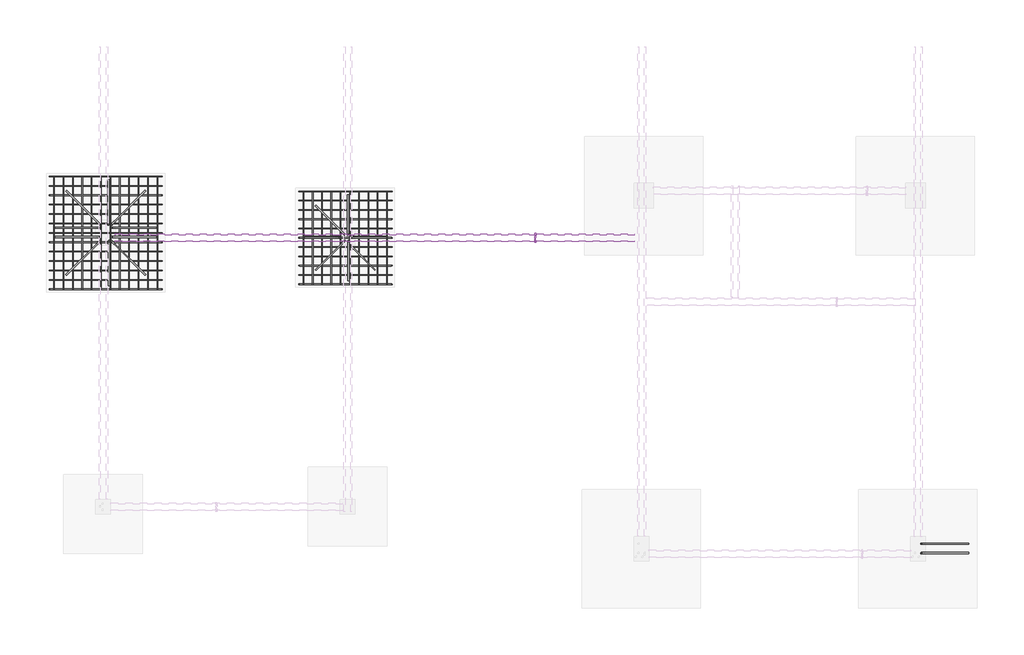
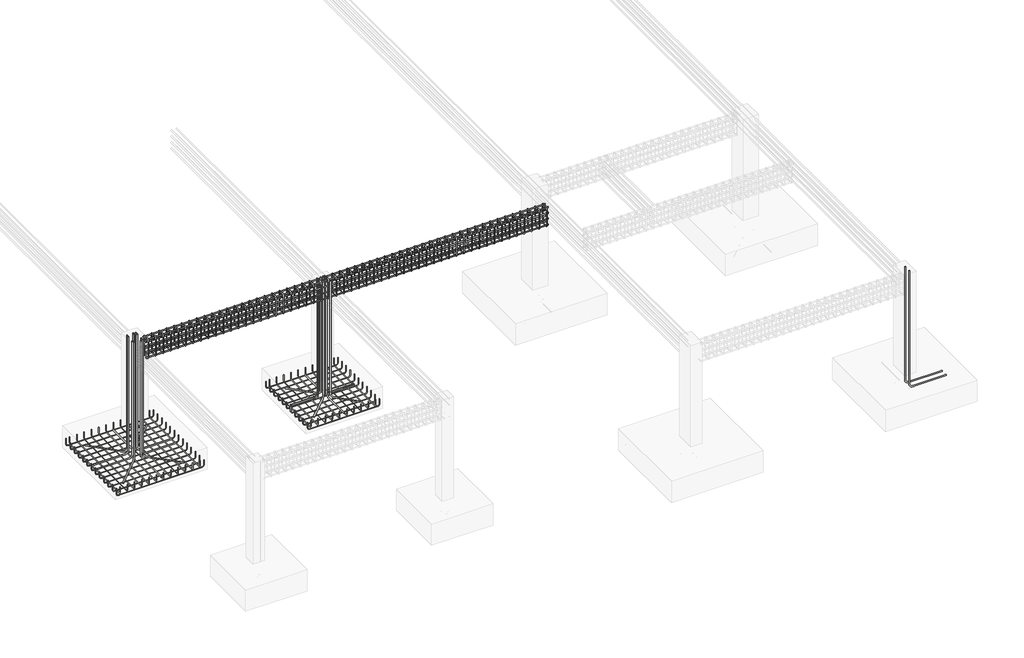
# One storey, part 4 of 10: 28 reinforcing bars.
"""IFC4 building model written with IfcOpenShell, lengths in millimetres."""

from ifc_helpers import new_model, si_unit, point, frame, origin, place, context, project, spatial, polyline, circle_curve, trimmed, segment, composite_curve, source, transform, mapped, element, save
from ifc_brep_helpers import swept_disk

model = new_model("IFC4")

# Units and contexts
model_context = context("Model", 3, world=origin())
ifc_project = project(units=[si_unit("LENGTHUNIT", "METRE", prefix="MILLI")], contexts=[model_context])

# Site, building, storey
site = spatial("IfcSite", under=ifc_project)
building = spatial("IfcBuilding", under=site)
storey = spatial("IfcBuildingStorey", under=building, Elevation=-2133.6)

# Reinforcing bars
placement = place(None, origin())
reinforcing_bar_shape = source(origin(), model_context, "Body", "SolidModel", [
    swept_disk(composite_curve([segment(polyline([(-4027.5164362, 1780.9219177, -2393.6), (-4027.5164362, 1780.9219177, -2504.1)]), True, "CONTINUOUS"), segment(trimmed(circle_curve(frame((-4062.2664362, 1780.9219177, -2504.1), z_axis=(0.0, 1.0, 0.0), x_axis=(34.75, 0.0, 0.0)), 34.75), [point((-4027.5164362, 1780.9219177, -2504.1))], [point((-4062.2664362, 1780.9219177, -2538.85))], True, "CARTESIAN"), True, "CONTINUOUS"), segment(polyline([(-4062.2664362, 1780.9219177, -2538.85), (-5732.0664362, 1780.9219177, -2538.85)]), True, "CONTINUOUS"), segment(trimmed(circle_curve(frame((-5732.0664362, 1780.9219177, -2504.1), z_axis=(0.0, 1.0, 0.0), x_axis=(0.0, 0.0, -34.75)), 34.75), [point((-5732.0664362, 1780.9219177, -2538.85))], [point((-5766.8164362, 1780.9219177, -2504.1))], True, "CARTESIAN"), True, "CONTINUOUS"), segment(polyline([(-5766.8164362, 1780.9219177, -2504.1), (-5766.8164362, 1780.9219177, -2393.6)]), True, "CONTINUOUS")], self_intersect=False), 4.75),
])
element("IfcReinforcingBar", 1, at=placement, inside=storey, context=model_context, shape_type="MappedRepresentation", body=[
    mapped(reinforcing_bar_shape, transform((0.0, 0.0, 0.0), x_axis=(1.0, 0.0, 0.0), y_axis=(0.0, 1.0, 0.0), z_axis=(0.0, 0.0, 1.0))),
    mapped(reinforcing_bar_shape, transform((0.0, -144.9416667, 0.0), x_axis=(1.0, 0.0, 0.0), y_axis=(0.0, 1.0, 0.0), z_axis=(0.0, 0.0, 1.0))),
    mapped(reinforcing_bar_shape, transform((0.0, -289.8833333, 0.0), x_axis=(1.0, 0.0, 0.0), y_axis=(0.0, 1.0, 0.0), z_axis=(0.0, 0.0, 1.0))),
    mapped(reinforcing_bar_shape, transform((0.0, -434.825, 0.0), x_axis=(1.0, 0.0, 0.0), y_axis=(0.0, 1.0, 0.0), z_axis=(0.0, 0.0, 1.0))),
    mapped(reinforcing_bar_shape, transform((0.0, -579.7666667, 0.0), x_axis=(1.0, 0.0, 0.0), y_axis=(0.0, 1.0, 0.0), z_axis=(0.0, 0.0, 1.0))),
    mapped(reinforcing_bar_shape, transform((0.0, -724.7083333, 0.0), x_axis=(1.0, 0.0, 0.0), y_axis=(0.0, 1.0, 0.0), z_axis=(0.0, 0.0, 1.0))),
    mapped(reinforcing_bar_shape, transform((0.0, -869.65, 0.0), x_axis=(1.0, 0.0, 0.0), y_axis=(0.0, 1.0, 0.0), z_axis=(0.0, 0.0, 1.0))),
    mapped(reinforcing_bar_shape, transform((0.0, -1014.5916667, 0.0), x_axis=(1.0, 0.0, 0.0), y_axis=(0.0, 1.0, 0.0), z_axis=(0.0, 0.0, 1.0))),
    mapped(reinforcing_bar_shape, transform((0.0, -1159.5333333, 0.0), x_axis=(1.0, 0.0, 0.0), y_axis=(0.0, 1.0, 0.0), z_axis=(0.0, 0.0, 1.0))),
    mapped(reinforcing_bar_shape, transform((0.0, -1304.475, 0.0), x_axis=(1.0, 0.0, 0.0), y_axis=(0.0, 1.0, 0.0), z_axis=(0.0, 0.0, 1.0))),
    mapped(reinforcing_bar_shape, transform((0.0, -1449.4166667, 0.0), x_axis=(1.0, 0.0, 0.0), y_axis=(0.0, 1.0, 0.0), z_axis=(0.0, 0.0, 1.0))),
    mapped(reinforcing_bar_shape, transform((0.0, -1594.3583333, 0.0), x_axis=(1.0, 0.0, 0.0), y_axis=(0.0, 1.0, 0.0), z_axis=(0.0, 0.0, 1.0))),
    mapped(reinforcing_bar_shape, transform((0.0, -1739.3, 0.0), x_axis=(1.0, 0.0, 0.0), y_axis=(0.0, 1.0, 0.0), z_axis=(0.0, 0.0, 1.0))),
])
reinforcing_bar_2_shape = source(origin(), model_context, "Body", "SolidModel", [
    swept_disk(composite_curve([segment(polyline([(-4102.4743867, 41.6219177, -2379.223371), (-4102.4743867, 41.6219177, -2489.723371)]), True, "CONTINUOUS"), segment(trimmed(circle_curve(frame((-4102.4743867, 76.3719177, -2489.723371), z_axis=(1.0, 0.0, 0.0), x_axis=(0.0, -34.75, 0.0)), 34.75), [point((-4102.4743867, 41.6219177, -2489.723371))], [point((-4102.4743867, 76.3719177, -2524.473371))], True, "CARTESIAN"), True, "CONTINUOUS"), segment(polyline([(-4102.4743867, 76.3719177, -2524.473371), (-4102.4743867, 1746.1719177, -2524.473371)]), True, "CONTINUOUS"), segment(trimmed(circle_curve(frame((-4102.4743867, 1746.1719177, -2489.723371), z_axis=(1.0, 0.0, 0.0), x_axis=(0.0, 0.0, -34.75)), 34.75), [point((-4102.4743867, 1746.1719177, -2524.473371))], [point((-4102.4743867, 1780.9219177, -2489.723371))], True, "CARTESIAN"), True, "CONTINUOUS"), segment(polyline([(-4102.4743867, 1780.9219177, -2489.723371), (-4102.4743867, 1780.9219177, -2379.223371)]), True, "CONTINUOUS")], self_intersect=False), 4.75),
])
element("IfcReinforcingBar", 2, at=placement, inside=storey, context=model_context, shape_type="MappedRepresentation", body=[
    mapped(reinforcing_bar_2_shape, transform((0.0, 0.0, 0.0), x_axis=(1.0, 0.0, 0.0), y_axis=(0.0, 1.0, 0.0), z_axis=(0.0, 0.0, 1.0))),
    mapped(reinforcing_bar_2_shape, transform((-144.8323389, 0.0, 0.0), x_axis=(1.0, 0.0, 0.0), y_axis=(0.0, 1.0, 0.0), z_axis=(0.0, 0.0, 1.0))),
    mapped(reinforcing_bar_2_shape, transform((-289.6646779, 0.0, 0.0), x_axis=(1.0, 0.0, 0.0), y_axis=(0.0, 1.0, 0.0), z_axis=(0.0, 0.0, 1.0))),
    mapped(reinforcing_bar_2_shape, transform((-434.4970168, 0.0, 0.0), x_axis=(1.0, 0.0, 0.0), y_axis=(0.0, 1.0, 0.0), z_axis=(0.0, 0.0, 1.0))),
    mapped(reinforcing_bar_2_shape, transform((-579.3293558, 0.0, 0.0), x_axis=(1.0, 0.0, 0.0), y_axis=(0.0, 1.0, 0.0), z_axis=(0.0, 0.0, 1.0))),
    mapped(reinforcing_bar_2_shape, transform((-724.1616947, 0.0, 0.0), x_axis=(1.0, 0.0, 0.0), y_axis=(0.0, 1.0, 0.0), z_axis=(0.0, 0.0, 1.0))),
    mapped(reinforcing_bar_2_shape, transform((-868.9940337, 0.0, 0.0), x_axis=(1.0, 0.0, 0.0), y_axis=(0.0, 1.0, 0.0), z_axis=(0.0, 0.0, 1.0))),
    mapped(reinforcing_bar_2_shape, transform((-1013.8263726, 0.0, 0.0), x_axis=(1.0, 0.0, 0.0), y_axis=(0.0, 1.0, 0.0), z_axis=(0.0, 0.0, 1.0))),
    mapped(reinforcing_bar_2_shape, transform((-1158.6587116, 0.0, 0.0), x_axis=(1.0, 0.0, 0.0), y_axis=(0.0, 1.0, 0.0), z_axis=(0.0, 0.0, 1.0))),
    mapped(reinforcing_bar_2_shape, transform((-1303.4910505, 0.0, 0.0), x_axis=(1.0, 0.0, 0.0), y_axis=(0.0, 1.0, 0.0), z_axis=(0.0, 0.0, 1.0))),
    mapped(reinforcing_bar_2_shape, transform((-1448.3233895, 0.0, 0.0), x_axis=(1.0, 0.0, 0.0), y_axis=(0.0, 1.0, 0.0), z_axis=(0.0, 0.0, 1.0))),
    mapped(reinforcing_bar_2_shape, transform((-1593.1557284, 0.0, 0.0), x_axis=(1.0, 0.0, 0.0), y_axis=(0.0, 1.0, 0.0), z_axis=(0.0, 0.0, 1.0))),
])
reinforcing_bar_3_shape = source(origin(), model_context, "Body", "SolidModel", [
    swept_disk(composite_curve([segment(polyline([(-484.2164362, 1552.3219177, -2393.6), (-484.2164362, 1552.3219177, -2504.1)]), True, "CONTINUOUS"), segment(trimmed(circle_curve(frame((-518.9664362, 1552.3219177, -2504.1), z_axis=(0.0, 1.0, 0.0), x_axis=(34.75, 0.0, 0.0)), 34.75), [point((-484.2164362, 1552.3219177, -2504.1))], [point((-518.9664362, 1552.3219177, -2538.85))], True, "CARTESIAN"), True, "CONTINUOUS"), segment(polyline([(-518.9664362, 1552.3219177, -2538.85), (-1883.9664362, 1552.3219177, -2538.85)]), True, "CONTINUOUS"), segment(trimmed(circle_curve(frame((-1883.9664362, 1552.3219177, -2504.1), z_axis=(0.0, 1.0, 0.0), x_axis=(0.0, 0.0, -34.75)), 34.75), [point((-1883.9664362, 1552.3219177, -2538.85))], [point((-1918.7164362, 1552.3219177, -2504.1))], True, "CARTESIAN"), True, "CONTINUOUS"), segment(polyline([(-1918.7164362, 1552.3219177, -2504.1), (-1918.7164362, 1552.3219177, -2393.6)]), True, "CONTINUOUS")], self_intersect=False), 4.75),
])
element("IfcReinforcingBar", 3, at=placement, inside=storey, context=model_context, shape_type="MappedRepresentation", body=[
    mapped(reinforcing_bar_3_shape, transform((0.0, 0.0, 0.0), x_axis=(1.0, 0.0, 0.0), y_axis=(0.0, 1.0, 0.0), z_axis=(0.0, 0.0, 1.0))),
    mapped(reinforcing_bar_3_shape, transform((0.0, -143.45, 0.0), x_axis=(1.0, 0.0, 0.0), y_axis=(0.0, 1.0, 0.0), z_axis=(0.0, 0.0, 1.0))),
    mapped(reinforcing_bar_3_shape, transform((0.0, -286.9, 0.0), x_axis=(1.0, 0.0, 0.0), y_axis=(0.0, 1.0, 0.0), z_axis=(0.0, 0.0, 1.0))),
    mapped(reinforcing_bar_3_shape, transform((0.0, -430.35, 0.0), x_axis=(1.0, 0.0, 0.0), y_axis=(0.0, 1.0, 0.0), z_axis=(0.0, 0.0, 1.0))),
    mapped(reinforcing_bar_3_shape, transform((0.0, -573.8, 0.0), x_axis=(1.0, 0.0, 0.0), y_axis=(0.0, 1.0, 0.0), z_axis=(0.0, 0.0, 1.0))),
    mapped(reinforcing_bar_3_shape, transform((0.0, -717.25, 0.0), x_axis=(1.0, 0.0, 0.0), y_axis=(0.0, 1.0, 0.0), z_axis=(0.0, 0.0, 1.0))),
    mapped(reinforcing_bar_3_shape, transform((0.0, -860.7, 0.0), x_axis=(1.0, 0.0, 0.0), y_axis=(0.0, 1.0, 0.0), z_axis=(0.0, 0.0, 1.0))),
    mapped(reinforcing_bar_3_shape, transform((0.0, -1004.15, 0.0), x_axis=(1.0, 0.0, 0.0), y_axis=(0.0, 1.0, 0.0), z_axis=(0.0, 0.0, 1.0))),
    mapped(reinforcing_bar_3_shape, transform((0.0, -1147.6, 0.0), x_axis=(1.0, 0.0, 0.0), y_axis=(0.0, 1.0, 0.0), z_axis=(0.0, 0.0, 1.0))),
    mapped(reinforcing_bar_3_shape, transform((0.0, -1291.05, 0.0), x_axis=(1.0, 0.0, 0.0), y_axis=(0.0, 1.0, 0.0), z_axis=(0.0, 0.0, 1.0))),
    mapped(reinforcing_bar_3_shape, transform((0.0, -1434.5, 0.0), x_axis=(1.0, 0.0, 0.0), y_axis=(0.0, 1.0, 0.0), z_axis=(0.0, 0.0, 1.0))),
])
reinforcing_bar_4_shape = source(origin(), model_context, "Body", "SolidModel", [
    swept_disk(composite_curve([segment(polyline([(-559.1743867, 117.8219177, -2379.223371), (-559.1743867, 117.8219177, -2489.723371)]), True, "CONTINUOUS"), segment(trimmed(circle_curve(frame((-559.1743867, 152.5719177, -2489.723371), z_axis=(1.0, 0.0, 0.0), x_axis=(0.0, -34.75, 0.0)), 34.75), [point((-559.1743867, 117.8219177, -2489.723371))], [point((-559.1743867, 152.5719177, -2524.473371))], True, "CARTESIAN"), True, "CONTINUOUS"), segment(polyline([(-559.1743867, 152.5719177, -2524.473371), (-559.1743867, 1517.5719177, -2524.473371)]), True, "CONTINUOUS"), segment(trimmed(circle_curve(frame((-559.1743867, 1517.5719177, -2489.723371), z_axis=(1.0, 0.0, 0.0), x_axis=(0.0, 0.0, -34.75)), 34.75), [point((-559.1743867, 1517.5719177, -2524.473371))], [point((-559.1743867, 1552.3219177, -2489.723371))], True, "CARTESIAN"), True, "CONTINUOUS"), segment(polyline([(-559.1743867, 1552.3219177, -2489.723371), (-559.1743867, 1552.3219177, -2379.223371)]), True, "CONTINUOUS")], self_intersect=False), 4.75),
])
element("IfcReinforcingBar", 4, at=placement, inside=storey, context=model_context, shape_type="MappedRepresentation", body=[
    mapped(reinforcing_bar_4_shape, transform((0.0, 0.0, 0.0), x_axis=(1.0, 0.0, 0.0), y_axis=(0.0, 1.0, 0.0), z_axis=(0.0, 0.0, 1.0))),
    mapped(reinforcing_bar_4_shape, transform((-143.1506365, 0.0, 0.0), x_axis=(1.0, 0.0, 0.0), y_axis=(0.0, 1.0, 0.0), z_axis=(0.0, 0.0, 1.0))),
    mapped(reinforcing_bar_4_shape, transform((-286.301273, 0.0, 0.0), x_axis=(1.0, 0.0, 0.0), y_axis=(0.0, 1.0, 0.0), z_axis=(0.0, 0.0, 1.0))),
    mapped(reinforcing_bar_4_shape, transform((-429.4519095, 0.0, 0.0), x_axis=(1.0, 0.0, 0.0), y_axis=(0.0, 1.0, 0.0), z_axis=(0.0, 0.0, 1.0))),
    mapped(reinforcing_bar_4_shape, transform((-572.602546, 0.0, 0.0), x_axis=(1.0, 0.0, 0.0), y_axis=(0.0, 1.0, 0.0), z_axis=(0.0, 0.0, 1.0))),
    mapped(reinforcing_bar_4_shape, transform((-715.7531825, 0.0, 0.0), x_axis=(1.0, 0.0, 0.0), y_axis=(0.0, 1.0, 0.0), z_axis=(0.0, 0.0, 1.0))),
    mapped(reinforcing_bar_4_shape, transform((-858.903819, 0.0, 0.0), x_axis=(1.0, 0.0, 0.0), y_axis=(0.0, 1.0, 0.0), z_axis=(0.0, 0.0, 1.0))),
    mapped(reinforcing_bar_4_shape, transform((-1002.0544555, 0.0, 0.0), x_axis=(1.0, 0.0, 0.0), y_axis=(0.0, 1.0, 0.0), z_axis=(0.0, 0.0, 1.0))),
    mapped(reinforcing_bar_4_shape, transform((-1145.205092, 0.0, 0.0), x_axis=(1.0, 0.0, 0.0), y_axis=(0.0, 1.0, 0.0), z_axis=(0.0, 0.0, 1.0))),
    mapped(reinforcing_bar_4_shape, transform((-1288.3557284, 0.0, 0.0), x_axis=(1.0, 0.0, 0.0), y_axis=(0.0, 1.0, 0.0), z_axis=(0.0, 0.0, 1.0))),
])
element("IfcReinforcingBar", 5, at=placement, inside=storey, context=model_context, shape_type="SolidModel", body=[
    swept_disk(composite_curve([segment(polyline([(-1210.5664362, 883.1552961, -40.0), (-1210.5664362, 883.1552961, -2426.55)]), True, "CONTINUOUS"), segment(trimmed(circle_curve(frame((-1257.9779458, 930.5668058, -2426.55), z_axis=(0.7071067811865519, 0.7071067811865431, 0.0), x_axis=(47.411509600000045, -47.41150970000001, 0.0)), 67.05), [point((-1210.5664362, 883.1552961, -2426.55))], [point((-1257.9779458, 930.5668058, -2493.6))], True, "CARTESIAN"), True, "CONTINUOUS"), segment(polyline([(-1257.9779458, 930.5668058, -2493.6), (-1658.7883692, 1331.3772292, -2493.6)]), True, "CONTINUOUS")], self_intersect=False), 9.55),
])
element("IfcReinforcingBar", 6, at=placement, inside=storey, context=model_context, shape_type="SolidModel", body=[
    swept_disk(composite_curve([segment(polyline([(-1210.5664362, 786.9885393, -40.0), (-1210.5664362, 786.9885393, -2426.55)]), True, "CONTINUOUS"), segment(trimmed(circle_curve(frame((-1257.9779458, 739.5770296, -2426.55), z_axis=(-0.7071067811865519, 0.7071067811865431, 0.0), x_axis=(47.411509600000045, 47.41150970000001, 0.0)), 67.05), [point((-1210.5664362, 786.9885393, -2426.55))], [point((-1257.9779458, 739.5770296, -2493.6))], True, "CARTESIAN"), True, "CONTINUOUS"), segment(polyline([(-1257.9779458, 739.5770296, -2493.6), (-1658.7883692, 338.7666062, -2493.6)]), True, "CONTINUOUS")], self_intersect=False), 9.55),
])
element("IfcReinforcingBar", 7, at=placement, inside=storey, context=model_context, shape_type="SolidModel", body=[
    swept_disk(composite_curve([segment(polyline([(-1115.0664362, 710.7885393, -40.0), (-1115.0664362, 710.7885393, -2426.55)]), True, "CONTINUOUS"), segment(trimmed(circle_curve(frame((-1067.6549265, 663.3770296, -2426.55), z_axis=(-0.7071067811865519, -0.7071067811865431, 0.0), x_axis=(-47.4115096999999, 47.41150970000001, 0.0)), 67.05), [point((-1115.0664362, 710.7885393, -2426.55))], [point((-1067.6549265, 663.3770296, -2493.6))], True, "CARTESIAN"), True, "CONTINUOUS"), segment(polyline([(-1067.6549265, 663.3770296, -2493.6), (-743.0445031, 338.7666062, -2493.6)]), True, "CONTINUOUS")], self_intersect=False), 9.55),
])
element("IfcReinforcingBar", 8, at=placement, inside=storey, context=model_context, shape_type="SolidModel", body=[
    swept_disk(composite_curve([segment(polyline([(-1161.6805145, 883.1552961, -40.0), (-1161.6805145, 883.1552961, -2426.55)]), True, "CONTINUOUS"), segment(trimmed(circle_curve(frame((-1161.6805145, 950.2052961, -2426.55), z_axis=(1.0, 0.0, 0.0), x_axis=(0.0, -67.05000000000007, 0.0)), 67.05), [point((-1161.6805145, 883.1552961, -2426.55))], [point((-1161.6805145, 950.2052961, -2493.6))], True, "CARTESIAN"), True, "CONTINUOUS"), segment(polyline([(-1161.6805145, 950.2052961, -2493.6), (-1161.6805145, 1501.2552961, -2493.6)]), True, "CONTINUOUS")], self_intersect=False), 9.55),
])
element("IfcReinforcingBar", 9, at=placement, inside=storey, context=model_context, shape_type="SolidModel", body=[
    swept_disk(composite_curve([segment(polyline([(-1151.6805145, 786.9885393, -40.0), (-1151.6805145, 786.9885393, -2426.55)]), True, "CONTINUOUS"), segment(trimmed(circle_curve(frame((-1151.6805145, 719.9385393, -2426.55), z_axis=(-1.0, 0.0, 0.0), x_axis=(0.0, 67.04999999999995, 0.0)), 67.05), [point((-1151.6805145, 786.9885393, -2426.55))], [point((-1151.6805145, 719.9385393, -2493.6))], True, "CARTESIAN"), True, "CONTINUOUS"), segment(polyline([(-1151.6805145, 719.9385393, -2493.6), (-1151.6805145, 168.8885393, -2493.6)]), True, "CONTINUOUS")], self_intersect=False), 9.55),
])
element("IfcReinforcingBar", 10, at=placement, inside=storey, context=model_context, shape_type="SolidModel", body=[
    swept_disk(composite_curve([segment(polyline([(-1286.7664362, 838.1552961, -40.0), (-1286.7664362, 838.1552961, -2426.55)]), True, "CONTINUOUS"), segment(trimmed(circle_curve(frame((-1353.8164362, 838.1552961, -2426.55), z_axis=(0.0, 1.0, 0.0), x_axis=(67.04999999999995, 0.0, 0.0)), 67.05), [point((-1286.7664362, 838.1552961, -2426.55))], [point((-1353.8164362, 838.1552961, -2493.6))], True, "CARTESIAN"), True, "CONTINUOUS"), segment(polyline([(-1353.8164362, 838.1552961, -2493.6), (-1828.6664362, 838.1552961, -2493.6)]), True, "CONTINUOUS")], self_intersect=False), 9.55),
])
element("IfcReinforcingBar", 11, at=placement, inside=storey, context=model_context, shape_type="SolidModel", body=[
    swept_disk(composite_curve([segment(polyline([(-1286.7664362, 847.2170998, -40.0), (-1286.7664362, 847.2170998, -2426.55)]), True, "CONTINUOUS"), segment(trimmed(circle_curve(frame((-1353.8164362, 847.2170998, -2426.55), z_axis=(0.0, 1.0, 0.0), x_axis=(67.04999999999995, 0.0, 0.0)), 67.05), [point((-1286.7664362, 847.2170998, -2426.55))], [point((-1353.8164362, 847.2170998, -2493.6))], True, "CARTESIAN"), True, "CONTINUOUS"), segment(polyline([(-1353.8164362, 847.2170998, -2493.6), (-1828.6664362, 847.2170998, -2493.6)]), True, "CONTINUOUS")], self_intersect=False), 9.55),
])
element("IfcReinforcingBar", 12, at=placement, inside=storey, context=model_context, shape_type="SolidModel", body=[
    swept_disk(composite_curve([segment(polyline([(-1115.0664362, 838.1552961, -40.0), (-1115.0664362, 838.1552961, -2426.55)]), True, "CONTINUOUS"), segment(trimmed(circle_curve(frame((-1048.0164362, 838.1552961, -2426.55), z_axis=(0.0, -1.0, 0.0), x_axis=(-67.04999999999995, 0.0, 0.0)), 67.05), [point((-1115.0664362, 838.1552961, -2426.55))], [point((-1048.0164362, 838.1552961, -2493.6))], True, "CARTESIAN"), True, "CONTINUOUS"), segment(polyline([(-1048.0164362, 838.1552961, -2493.6), (-573.1664362, 838.1552961, -2493.6)]), True, "CONTINUOUS")], self_intersect=False), 9.55),
])
element("IfcReinforcingBar", 13, at=placement, inside=storey, context=model_context, shape_type="SolidModel", body=[
    swept_disk(composite_curve([segment(polyline([(-1115.0664362, 847.2170998, -40.0), (-1115.0664362, 847.2170998, -2426.55)]), True, "CONTINUOUS"), segment(trimmed(circle_curve(frame((-1048.0164362, 847.2170998, -2426.55), z_axis=(0.0, -1.0, 0.0), x_axis=(-67.04999999999995, 0.0, 0.0)), 67.05), [point((-1115.0664362, 847.2170998, -2426.55))], [point((-1048.0164362, 847.2170998, -2493.6))], True, "CARTESIAN"), True, "CONTINUOUS"), segment(polyline([(-1048.0164362, 847.2170998, -2493.6), (-573.1664362, 847.2170998, -2493.6)]), True, "CONTINUOUS")], self_intersect=False), 9.55),
])
element("IfcReinforcingBar", 14, at=placement, inside=storey, context=model_context, shape_type="SolidModel", body=[
    swept_disk(composite_curve([segment(polyline([(-4982.4664362, 1035.5552961, -40.0), (-4982.4664362, 1035.5552961, -2426.55)]), True, "CONTINUOUS"), segment(trimmed(circle_curve(frame((-5029.8779458, 1082.9668058, -2426.55), z_axis=(0.7071067811865519, 0.7071067811865431, 0.0), x_axis=(47.41150959999959, -47.4115096999999, 0.0)), 67.05), [point((-4982.4664362, 1035.5552961, -2426.55))], [point((-5029.8779458, 1082.9668058, -2493.6))], True, "CARTESIAN"), True, "CONTINUOUS"), segment(polyline([(-5029.8779458, 1082.9668058, -2493.6), (-5506.8883692, 1559.9772292, -2493.6)]), True, "CONTINUOUS")], self_intersect=False), 9.55),
])
element("IfcReinforcingBar", 15, at=placement, inside=storey, context=model_context, shape_type="SolidModel", body=[
    swept_disk(composite_curve([segment(polyline([(-4810.7664362, 1035.5552961, -40.0), (-4810.7664362, 1035.5552961, -2426.55)]), True, "CONTINUOUS"), segment(trimmed(circle_curve(frame((-4763.3549265, 1082.9668058, -2426.55), z_axis=(0.7071067811865519, -0.7071067811865431, 0.0), x_axis=(-47.41150969999944, -47.4115096999999, 0.0)), 67.05), [point((-4810.7664362, 1035.5552961, -2426.55))], [point((-4763.3549265, 1082.9668058, -2493.6))], True, "CARTESIAN"), True, "CONTINUOUS"), segment(polyline([(-4763.3549265, 1082.9668058, -2493.6), (-4286.3445031, 1559.9772292, -2493.6)]), True, "CONTINUOUS")], self_intersect=False), 9.55),
])
element("IfcReinforcingBar", 16, at=placement, inside=storey, context=model_context, shape_type="SolidModel", body=[
    swept_disk(composite_curve([segment(polyline([(-4982.4664362, 786.9885393, -40.0), (-4982.4664362, 786.9885393, -2426.55)]), True, "CONTINUOUS"), segment(trimmed(circle_curve(frame((-5029.8779458, 739.5770296, -2426.55), z_axis=(-0.7071067811865519, 0.7071067811865431, 0.0), x_axis=(47.41150959999959, 47.41150970000001, 0.0)), 67.05), [point((-4982.4664362, 786.9885393, -2426.55))], [point((-5029.8779458, 739.5770296, -2493.6))], True, "CARTESIAN"), True, "CONTINUOUS"), segment(polyline([(-5029.8779458, 739.5770296, -2493.6), (-5506.8883692, 262.5666062, -2493.6)]), True, "CONTINUOUS")], self_intersect=False), 9.55),
])
element("IfcReinforcingBar", 17, at=placement, inside=storey, context=model_context, shape_type="SolidModel", body=[
    swept_disk(composite_curve([segment(polyline([(-4810.7664362, 786.9885393, -40.0), (-4810.7664362, 786.9885393, -2426.55)]), True, "CONTINUOUS"), segment(trimmed(circle_curve(frame((-4763.3549265, 739.5770296, -2426.55), z_axis=(-0.7071067811865519, -0.7071067811865431, 0.0), x_axis=(-47.41150969999944, 47.41150970000001, 0.0)), 67.05), [point((-4810.7664362, 786.9885393, -2426.55))], [point((-4763.3549265, 739.5770296, -2493.6))], True, "CARTESIAN"), True, "CONTINUOUS"), segment(polyline([(-4763.3549265, 739.5770296, -2493.6), (-4286.3445031, 262.5666062, -2493.6)]), True, "CONTINUOUS")], self_intersect=False), 9.55),
])
element("IfcReinforcingBar", 18, at=placement, inside=storey, context=model_context, shape_type="SolidModel", body=[
    swept_disk(composite_curve([segment(polyline([(-4857.3805145, 1035.5552961, -40.0), (-4857.3805145, 1035.5552961, -2426.55)]), True, "CONTINUOUS"), segment(trimmed(circle_curve(frame((-4857.3805145, 1102.6052961, -2426.55), z_axis=(1.0, 0.0, 0.0), x_axis=(0.0, -67.04999999999995, 0.0)), 67.05), [point((-4857.3805145, 1035.5552961, -2426.55))], [point((-4857.3805145, 1102.6052961, -2493.6))], True, "CARTESIAN"), True, "CONTINUOUS"), segment(polyline([(-4857.3805145, 1102.6052961, -2493.6), (-4857.3805145, 1729.8552961, -2493.6)]), True, "CONTINUOUS")], self_intersect=False), 9.55),
])
element("IfcReinforcingBar", 19, at=placement, inside=storey, context=model_context, shape_type="SolidModel", body=[
    swept_disk(composite_curve([segment(polyline([(-4847.3805145, 786.9885393, -40.0), (-4847.3805145, 786.9885393, -2426.55)]), True, "CONTINUOUS"), segment(trimmed(circle_curve(frame((-4847.3805145, 719.9385393, -2426.55), z_axis=(-1.0, 0.0, 0.0), x_axis=(0.0, 67.04999999999995, 0.0)), 67.05), [point((-4847.3805145, 786.9885393, -2426.55))], [point((-4847.3805145, 719.9385393, -2493.6))], True, "CARTESIAN"), True, "CONTINUOUS"), segment(polyline([(-4847.3805145, 719.9385393, -2493.6), (-4847.3805145, 92.6885393, -2493.6)]), True, "CONTINUOUS")], self_intersect=False), 9.55),
])
element("IfcReinforcingBar", 20, at=placement, inside=storey, context=model_context, shape_type="SolidModel", body=[
    swept_disk(composite_curve([segment(polyline([(-4982.4664362, 990.5552961, -40.0), (-4982.4664362, 990.5552961, -2426.55)]), True, "CONTINUOUS"), segment(trimmed(circle_curve(frame((-5049.5164362, 990.5552961, -2426.55), z_axis=(0.0, 1.0, 0.0), x_axis=(67.04999999999927, 0.0, 0.0)), 67.05), [point((-4982.4664362, 990.5552961, -2426.55))], [point((-5049.5164362, 990.5552961, -2493.6))], True, "CARTESIAN"), True, "CONTINUOUS"), segment(polyline([(-5049.5164362, 990.5552961, -2493.6), (-5676.7664362, 990.5552961, -2493.6)]), True, "CONTINUOUS")], self_intersect=False), 9.55),
])
element("IfcReinforcingBar", 21, at=placement, inside=storey, context=model_context, shape_type="SolidModel", body=[
    swept_disk(composite_curve([segment(polyline([(-4982.4664362, 847.2170998, -40.0), (-4982.4664362, 847.2170998, -2426.55)]), True, "CONTINUOUS"), segment(trimmed(circle_curve(frame((-5049.5164362, 847.2170998, -2426.55), z_axis=(0.0, 1.0, 0.0), x_axis=(67.04999999999927, 0.0, 0.0)), 67.05), [point((-4982.4664362, 847.2170998, -2426.55))], [point((-5049.5164362, 847.2170998, -2493.6))], True, "CARTESIAN"), True, "CONTINUOUS"), segment(polyline([(-5049.5164362, 847.2170998, -2493.6), (-5676.7664362, 847.2170998, -2493.6)]), True, "CONTINUOUS")], self_intersect=False), 9.55),
])
element("IfcReinforcingBar", 22, at=placement, inside=storey, context=model_context, shape_type="SolidModel", body=[
    swept_disk(composite_curve([segment(polyline([(-4810.7664362, 990.5552961, -40.0), (-4810.7664362, 990.5552961, -2426.55)]), True, "CONTINUOUS"), segment(trimmed(circle_curve(frame((-4743.7164362, 990.5552961, -2426.55), z_axis=(0.0, -1.0, 0.0), x_axis=(-67.04999999999927, 0.0, 0.0)), 67.05), [point((-4810.7664362, 990.5552961, -2426.55))], [point((-4743.7164362, 990.5552961, -2493.6))], True, "CARTESIAN"), True, "CONTINUOUS"), segment(polyline([(-4743.7164362, 990.5552961, -2493.6), (-4116.4664362, 990.5552961, -2493.6)]), True, "CONTINUOUS")], self_intersect=False), 9.55),
])
element("IfcReinforcingBar", 23, at=placement, inside=storey, context=model_context, shape_type="SolidModel", body=[
    swept_disk(composite_curve([segment(polyline([(-4810.7664362, 847.2170998, -40.0), (-4810.7664362, 847.2170998, -2426.55)]), True, "CONTINUOUS"), segment(trimmed(circle_curve(frame((-4743.7164362, 847.2170998, -2426.55), z_axis=(0.0, -1.0, 0.0), x_axis=(-67.04999999999927, 0.0, 0.0)), 67.05), [point((-4810.7664362, 847.2170998, -2426.55))], [point((-4743.7164362, 847.2170998, -2493.6))], True, "CARTESIAN"), True, "CONTINUOUS"), segment(polyline([(-4743.7164362, 847.2170998, -2493.6), (-4116.4664362, 847.2170998, -2493.6)]), True, "CONTINUOUS")], self_intersect=False), 9.55),
])
element("IfcReinforcingBar", 24, at=placement, inside=storey, context=model_context, shape_type="SolidModel", body=[
    swept_disk(composite_curve([segment(polyline([(7686.0335638, -3886.2447039, -40.0), (7686.0335638, -3886.2447039, -2426.55)]), True, "CONTINUOUS"), segment(trimmed(circle_curve(frame((7753.0835638, -3886.2447039, -2426.55), z_axis=(0.0, -1.0, 0.0), x_axis=(-67.05000000000018, 0.0, 0.0)), 67.05), [point((7686.0335638, -3886.2447039, -2426.55))], [point((7753.0835638, -3886.2447039, -2493.6))], True, "CARTESIAN"), True, "CONTINUOUS"), segment(polyline([(7753.0835638, -3886.2447039, -2493.6), (8418.4335638, -3886.2447039, -2493.6)]), True, "CONTINUOUS")], self_intersect=False), 9.55),
])
element("IfcReinforcingBar", 25, at=placement, inside=storey, context=model_context, shape_type="SolidModel", body=[
    swept_disk(composite_curve([segment(polyline([(7686.0335638, -4029.5829002, -40.0), (7686.0335638, -4029.5829002, -2426.55)]), True, "CONTINUOUS"), segment(trimmed(circle_curve(frame((7753.0835638, -4029.5829002, -2426.55), z_axis=(0.0, -1.0, 0.0), x_axis=(-67.05000000000018, 0.0, 0.0)), 67.05), [point((7686.0335638, -4029.5829002, -2426.55))], [point((7753.0835638, -4029.5829002, -2493.6))], True, "CARTESIAN"), True, "CONTINUOUS"), segment(polyline([(7753.0835638, -4029.5829002, -2493.6), (8418.4335638, -4029.5829002, -2493.6)]), True, "CONTINUOUS")], self_intersect=False), 9.55),
])
reinforcing_bar_5_shape = source(origin(), model_context, "Body", "SolidModel", [
    swept_disk(composite_curve([segment(polyline([(-4713.4921956, 865.1786993, -109.4049959), (-4713.4921956, 807.7728105, -51.9991072)]), True, "CONTINUOUS"), segment(trimmed(circle_curve(frame((-4713.4921956, 790.2719177, -69.5), z_axis=(1.0, 0.0, 0.0), x_axis=(0.0, 17.500892799999974, 17.500892800000003)), 24.75), [point((-4713.4921956, 807.7728105, -51.9991072))], [point((-4713.4921956, 765.5219177, -69.5))], True, "CARTESIAN"), True, "CONTINUOUS"), segment(polyline([(-4713.4921956, 765.5219177, -69.5), (-4713.4921956, 765.5219177, -430.5)]), True, "CONTINUOUS"), segment(trimmed(circle_curve(frame((-4713.4921956, 790.2719177, -430.5), z_axis=(1.0, 0.0, 0.0), x_axis=(0.0, -24.75, 0.0)), 24.75), [point((-4713.4921956, 765.5219177, -430.5))], [point((-4713.4921956, 790.2719177, -455.25))], True, "CARTESIAN"), True, "CONTINUOUS"), segment(polyline([(-4713.4921956, 790.2719177, -455.25), (-4713.4921956, 879.8719177, -455.25)]), True, "CONTINUOUS"), segment(trimmed(circle_curve(frame((-4714.0648194, 879.8719177, -430.5066251), z_axis=(0.9997323196529888, 0.0, 0.02313631434032496), x_axis=(0.5726237999997466, 0.0, -24.743374899999992)), 24.75), [point((-4713.4921956, 879.8719177, -455.25))], [point((-4714.0648194, 904.6219177, -430.5066251))], True, "CARTESIAN"), True, "CONTINUOUS"), segment(polyline([(-4714.0648194, 904.6219177, -430.5066251), (-4722.4195719, 904.6219177, -69.4933749)]), True, "CONTINUOUS"), segment(trimmed(circle_curve(frame((-4722.4195719, 879.8719177, -69.4933749), z_axis=(0.9997323196529888, 0.0, 0.02313631434032496), x_axis=(0.0, 24.75, 0.0)), 24.75), [point((-4722.4195719, 904.6219177, -69.4933749))], [point((-4722.9921956, 879.8719177, -44.75))], True, "CARTESIAN"), True, "CONTINUOUS"), segment(polyline([(-4722.9921956, 879.8719177, -44.75), (-4722.9921956, 790.2719177, -44.75)]), True, "CONTINUOUS"), segment(trimmed(circle_curve(frame((-4722.9921956, 790.2719177, -69.5), z_axis=(1.0, 0.0, 0.0), x_axis=(0.0, 0.0, 24.75)), 24.75), [point((-4722.9921956, 790.2719177, -44.75))], [point((-4722.9921956, 772.7710249, -87.0008928))], True, "CARTESIAN"), True, "CONTINUOUS"), segment(polyline([(-4722.9921956, 772.7710249, -87.0008928), (-4722.9921956, 830.1769136, -144.4067815)]), True, "CONTINUOUS")], self_intersect=False), 4.75),
])
element("IfcReinforcingBar", 26, at=placement, inside=storey, context=model_context, shape_type="MappedRepresentation", body=[
    mapped(reinforcing_bar_5_shape, transform((0.0, 0.0, 0.0), x_axis=(1.0, 0.0, 0.0), y_axis=(0.0, 1.0, 0.0), z_axis=(0.0, 0.0, 1.0))),
    mapped(reinforcing_bar_5_shape, transform((149.9076675, 0.0, 0.0), x_axis=(1.0, 0.0, 0.0), y_axis=(0.0, 1.0, 0.0), z_axis=(0.0, 0.0, 1.0))),
    mapped(reinforcing_bar_5_shape, transform((299.8153351, 0.0, 0.0), x_axis=(1.0, 0.0, 0.0), y_axis=(0.0, 1.0, 0.0), z_axis=(0.0, 0.0, 1.0))),
    mapped(reinforcing_bar_5_shape, transform((449.7230026, 0.0, 0.0), x_axis=(1.0, 0.0, 0.0), y_axis=(0.0, 1.0, 0.0), z_axis=(0.0, 0.0, 1.0))),
    mapped(reinforcing_bar_5_shape, transform((599.6306702, 0.0, 0.0), x_axis=(1.0, 0.0, 0.0), y_axis=(0.0, 1.0, 0.0), z_axis=(0.0, 0.0, 1.0))),
    mapped(reinforcing_bar_5_shape, transform((749.5383377, 0.0, 0.0), x_axis=(1.0, 0.0, 0.0), y_axis=(0.0, 1.0, 0.0), z_axis=(0.0, 0.0, 1.0))),
    mapped(reinforcing_bar_5_shape, transform((899.4460053, 0.0, 0.0), x_axis=(1.0, 0.0, 0.0), y_axis=(0.0, 1.0, 0.0), z_axis=(0.0, 0.0, 1.0))),
    mapped(reinforcing_bar_5_shape, transform((1049.3536728, 0.0, 0.0), x_axis=(1.0, 0.0, 0.0), y_axis=(0.0, 1.0, 0.0), z_axis=(0.0, 0.0, 1.0))),
    mapped(reinforcing_bar_5_shape, transform((1199.2613404, 0.0, 0.0), x_axis=(1.0, 0.0, 0.0), y_axis=(0.0, 1.0, 0.0), z_axis=(0.0, 0.0, 1.0))),
    mapped(reinforcing_bar_5_shape, transform((1349.1690079, 0.0, 0.0), x_axis=(1.0, 0.0, 0.0), y_axis=(0.0, 1.0, 0.0), z_axis=(0.0, 0.0, 1.0))),
    mapped(reinforcing_bar_5_shape, transform((1499.0766755, 0.0, 0.0), x_axis=(1.0, 0.0, 0.0), y_axis=(0.0, 1.0, 0.0), z_axis=(0.0, 0.0, 1.0))),
    mapped(reinforcing_bar_5_shape, transform((1648.984343, 0.0, 0.0), x_axis=(1.0, 0.0, 0.0), y_axis=(0.0, 1.0, 0.0), z_axis=(0.0, 0.0, 1.0))),
    mapped(reinforcing_bar_5_shape, transform((1798.8920106, 0.0, 0.0), x_axis=(1.0, 0.0, 0.0), y_axis=(0.0, 1.0, 0.0), z_axis=(0.0, 0.0, 1.0))),
    mapped(reinforcing_bar_5_shape, transform((1948.7996781, 0.0, 0.0), x_axis=(1.0, 0.0, 0.0), y_axis=(0.0, 1.0, 0.0), z_axis=(0.0, 0.0, 1.0))),
    mapped(reinforcing_bar_5_shape, transform((2098.7073457, 0.0, 0.0), x_axis=(1.0, 0.0, 0.0), y_axis=(0.0, 1.0, 0.0), z_axis=(0.0, 0.0, 1.0))),
    mapped(reinforcing_bar_5_shape, transform((2248.6150132, 0.0, 0.0), x_axis=(1.0, 0.0, 0.0), y_axis=(0.0, 1.0, 0.0), z_axis=(0.0, 0.0, 1.0))),
    mapped(reinforcing_bar_5_shape, transform((2398.5226808, 0.0, 0.0), x_axis=(1.0, 0.0, 0.0), y_axis=(0.0, 1.0, 0.0), z_axis=(0.0, 0.0, 1.0))),
    mapped(reinforcing_bar_5_shape, transform((2548.4303483, 0.0, 0.0), x_axis=(1.0, 0.0, 0.0), y_axis=(0.0, 1.0, 0.0), z_axis=(0.0, 0.0, 1.0))),
    mapped(reinforcing_bar_5_shape, transform((2698.3380158, 0.0, 0.0), x_axis=(1.0, 0.0, 0.0), y_axis=(0.0, 1.0, 0.0), z_axis=(0.0, 0.0, 1.0))),
    mapped(reinforcing_bar_5_shape, transform((2848.2456834, 0.0, 0.0), x_axis=(1.0, 0.0, 0.0), y_axis=(0.0, 1.0, 0.0), z_axis=(0.0, 0.0, 1.0))),
    mapped(reinforcing_bar_5_shape, transform((2998.1533509, 0.0, 0.0), x_axis=(1.0, 0.0, 0.0), y_axis=(0.0, 1.0, 0.0), z_axis=(0.0, 0.0, 1.0))),
    mapped(reinforcing_bar_5_shape, transform((3148.0610185, 0.0, 0.0), x_axis=(1.0, 0.0, 0.0), y_axis=(0.0, 1.0, 0.0), z_axis=(0.0, 0.0, 1.0))),
    mapped(reinforcing_bar_5_shape, transform((3297.968686, 0.0, 0.0), x_axis=(1.0, 0.0, 0.0), y_axis=(0.0, 1.0, 0.0), z_axis=(0.0, 0.0, 1.0))),
    mapped(reinforcing_bar_5_shape, transform((3447.8763536, 0.0, 0.0), x_axis=(1.0, 0.0, 0.0), y_axis=(0.0, 1.0, 0.0), z_axis=(0.0, 0.0, 1.0))),
    mapped(reinforcing_bar_5_shape, transform((3597.7840211, 0.0, 0.0), x_axis=(1.0, 0.0, 0.0), y_axis=(0.0, 1.0, 0.0), z_axis=(0.0, 0.0, 1.0))),
    mapped(reinforcing_bar_5_shape, transform((3747.6916887, 0.0, 0.0), x_axis=(1.0, 0.0, 0.0), y_axis=(0.0, 1.0, 0.0), z_axis=(0.0, 0.0, 1.0))),
    mapped(reinforcing_bar_5_shape, transform((3897.5993562, 0.0, 0.0), x_axis=(1.0, 0.0, 0.0), y_axis=(0.0, 1.0, 0.0), z_axis=(0.0, 0.0, 1.0))),
    mapped(reinforcing_bar_5_shape, transform((4047.5070238, 0.0, 0.0), x_axis=(1.0, 0.0, 0.0), y_axis=(0.0, 1.0, 0.0), z_axis=(0.0, 0.0, 1.0))),
    mapped(reinforcing_bar_5_shape, transform((4197.4146913, 0.0, 0.0), x_axis=(1.0, 0.0, 0.0), y_axis=(0.0, 1.0, 0.0), z_axis=(0.0, 0.0, 1.0))),
    mapped(reinforcing_bar_5_shape, transform((4347.3223589, 0.0, 0.0), x_axis=(1.0, 0.0, 0.0), y_axis=(0.0, 1.0, 0.0), z_axis=(0.0, 0.0, 1.0))),
    mapped(reinforcing_bar_5_shape, transform((4497.2300264, 0.0, 0.0), x_axis=(1.0, 0.0, 0.0), y_axis=(0.0, 1.0, 0.0), z_axis=(0.0, 0.0, 1.0))),
    mapped(reinforcing_bar_5_shape, transform((4647.137694, 0.0, 0.0), x_axis=(1.0, 0.0, 0.0), y_axis=(0.0, 1.0, 0.0), z_axis=(0.0, 0.0, 1.0))),
    mapped(reinforcing_bar_5_shape, transform((4797.0453615, 0.0, 0.0), x_axis=(1.0, 0.0, 0.0), y_axis=(0.0, 1.0, 0.0), z_axis=(0.0, 0.0, 1.0))),
    mapped(reinforcing_bar_5_shape, transform((4946.9530291, 0.0, 0.0), x_axis=(1.0, 0.0, 0.0), y_axis=(0.0, 1.0, 0.0), z_axis=(0.0, 0.0, 1.0))),
    mapped(reinforcing_bar_5_shape, transform((5096.8606966, 0.0, 0.0), x_axis=(1.0, 0.0, 0.0), y_axis=(0.0, 1.0, 0.0), z_axis=(0.0, 0.0, 1.0))),
    mapped(reinforcing_bar_5_shape, transform((5246.7683642, 0.0, 0.0), x_axis=(1.0, 0.0, 0.0), y_axis=(0.0, 1.0, 0.0), z_axis=(0.0, 0.0, 1.0))),
    mapped(reinforcing_bar_5_shape, transform((5396.6760317, 0.0, 0.0), x_axis=(1.0, 0.0, 0.0), y_axis=(0.0, 1.0, 0.0), z_axis=(0.0, 0.0, 1.0))),
    mapped(reinforcing_bar_5_shape, transform((5546.5836992, 0.0, 0.0), x_axis=(1.0, 0.0, 0.0), y_axis=(0.0, 1.0, 0.0), z_axis=(0.0, 0.0, 1.0))),
    mapped(reinforcing_bar_5_shape, transform((5696.4913668, 0.0, 0.0), x_axis=(1.0, 0.0, 0.0), y_axis=(0.0, 1.0, 0.0), z_axis=(0.0, 0.0, 1.0))),
    mapped(reinforcing_bar_5_shape, transform((5846.3990343, 0.0, 0.0), x_axis=(1.0, 0.0, 0.0), y_axis=(0.0, 1.0, 0.0), z_axis=(0.0, 0.0, 1.0))),
    mapped(reinforcing_bar_5_shape, transform((5996.3067019, 0.0, 0.0), x_axis=(1.0, 0.0, 0.0), y_axis=(0.0, 1.0, 0.0), z_axis=(0.0, 0.0, 1.0))),
    mapped(reinforcing_bar_5_shape, transform((6146.2143694, 0.0, 0.0), x_axis=(1.0, 0.0, 0.0), y_axis=(0.0, 1.0, 0.0), z_axis=(0.0, 0.0, 1.0))),
    mapped(reinforcing_bar_5_shape, transform((6296.122037, 0.0, 0.0), x_axis=(1.0, 0.0, 0.0), y_axis=(0.0, 1.0, 0.0), z_axis=(0.0, 0.0, 1.0))),
    mapped(reinforcing_bar_5_shape, transform((6446.0297045, 0.0, 0.0), x_axis=(1.0, 0.0, 0.0), y_axis=(0.0, 1.0, 0.0), z_axis=(0.0, 0.0, 1.0))),
    mapped(reinforcing_bar_5_shape, transform((6595.9373721, 0.0, 0.0), x_axis=(1.0, 0.0, 0.0), y_axis=(0.0, 1.0, 0.0), z_axis=(0.0, 0.0, 1.0))),
    mapped(reinforcing_bar_5_shape, transform((6745.8450396, 0.0, 0.0), x_axis=(1.0, 0.0, 0.0), y_axis=(0.0, 1.0, 0.0), z_axis=(0.0, 0.0, 1.0))),
    mapped(reinforcing_bar_5_shape, transform((6895.7527072, 0.0, 0.0), x_axis=(1.0, 0.0, 0.0), y_axis=(0.0, 1.0, 0.0), z_axis=(0.0, 0.0, 1.0))),
    mapped(reinforcing_bar_5_shape, transform((7045.6603747, 0.0, 0.0), x_axis=(1.0, 0.0, 0.0), y_axis=(0.0, 1.0, 0.0), z_axis=(0.0, 0.0, 1.0))),
    mapped(reinforcing_bar_5_shape, transform((7195.5680423, 0.0, 0.0), x_axis=(1.0, 0.0, 0.0), y_axis=(0.0, 1.0, 0.0), z_axis=(0.0, 0.0, 1.0))),
    mapped(reinforcing_bar_5_shape, transform((7345.4757098, 0.0, 0.0), x_axis=(1.0, 0.0, 0.0), y_axis=(0.0, 1.0, 0.0), z_axis=(0.0, 0.0, 1.0))),
    mapped(reinforcing_bar_5_shape, transform((7495.3833774, 0.0, 0.0), x_axis=(1.0, 0.0, 0.0), y_axis=(0.0, 1.0, 0.0), z_axis=(0.0, 0.0, 1.0))),
    mapped(reinforcing_bar_5_shape, transform((7645.2910449, 0.0, 0.0), x_axis=(1.0, 0.0, 0.0), y_axis=(0.0, 1.0, 0.0), z_axis=(0.0, 0.0, 1.0))),
    mapped(reinforcing_bar_5_shape, transform((7795.1987125, 0.0, 0.0), x_axis=(1.0, 0.0, 0.0), y_axis=(0.0, 1.0, 0.0), z_axis=(0.0, 0.0, 1.0))),
    mapped(reinforcing_bar_5_shape, transform((7945.10638, 0.0, 0.0), x_axis=(1.0, 0.0, 0.0), y_axis=(0.0, 1.0, 0.0), z_axis=(0.0, 0.0, 1.0))),
])
reinforcing_bar_6_shape = source(origin(), model_context, "Body", "SolidModel", [
    swept_disk(composite_curve([segment(polyline([(-4750.5565806, 782.8826519, -62.1107341), (3265.2989804, 782.8826519, -62.1107341)]), True, "CONTINUOUS")], self_intersect=False), 9.55),
])
element("IfcReinforcingBar", 27, at=placement, inside=storey, context=model_context, shape_type="MappedRepresentation", body=[
    mapped(reinforcing_bar_6_shape, transform((0.0, 0.0, 0.0), x_axis=(1.0, 0.0, 0.0), y_axis=(0.0, 1.0, 0.0), z_axis=(0.0, 0.0, 1.0))),
    mapped(reinforcing_bar_6_shape, transform((0.0, 0.0, -125.2595106), x_axis=(1.0, 0.0, 0.0), y_axis=(0.0, 1.0, 0.0), z_axis=(0.0, 0.0, 1.0))),
    mapped(reinforcing_bar_6_shape, transform((0.0, 0.0, -250.5190212), x_axis=(1.0, 0.0, 0.0), y_axis=(0.0, 1.0, 0.0), z_axis=(0.0, 0.0, 1.0))),
    mapped(reinforcing_bar_6_shape, transform((0.0, 0.0, -375.7785317), x_axis=(1.0, 0.0, 0.0), y_axis=(0.0, 1.0, 0.0), z_axis=(0.0, 0.0, 1.0))),
])
reinforcing_bar_7_shape = source(origin(), model_context, "Body", "SolidModel", [
    swept_disk(composite_curve([segment(polyline([(-4748.2220523, 887.2611836, -62.1107341), (3264.2544813, 887.2611836, -62.1107341)]), True, "CONTINUOUS")], self_intersect=False), 9.55),
])
element("IfcReinforcingBar", 28, at=placement, inside=storey, context=model_context, shape_type="MappedRepresentation", body=[
    mapped(reinforcing_bar_7_shape, transform((0.0, 0.0, 0.0), x_axis=(1.0, 0.0, 0.0), y_axis=(0.0, 1.0, 0.0), z_axis=(0.0, 0.0, 1.0))),
    mapped(reinforcing_bar_7_shape, transform((0.0, 0.0, -125.2595106), x_axis=(1.0, 0.0, 0.0), y_axis=(0.0, 1.0, 0.0), z_axis=(0.0, 0.0, 1.0))),
    mapped(reinforcing_bar_7_shape, transform((0.0, 0.0, -250.5190212), x_axis=(1.0, 0.0, 0.0), y_axis=(0.0, 1.0, 0.0), z_axis=(0.0, 0.0, 1.0))),
    mapped(reinforcing_bar_7_shape, transform((0.0, 0.0, -375.7785317), x_axis=(1.0, 0.0, 0.0), y_axis=(0.0, 1.0, 0.0), z_axis=(0.0, 0.0, 1.0))),
])

save(model, "model.ifc")

# Revit data of these elements
# Elements 1, 2, 3, 4, 5, 6, 7, 8, 9, 10, 11, 12, 13, 14, 15, 16, 17, 18, 19, 20, 21, 22, 23, 24, 25, 26, 27, 28 (IfcReinforcingBar)
#   Phase Created = New Construction
